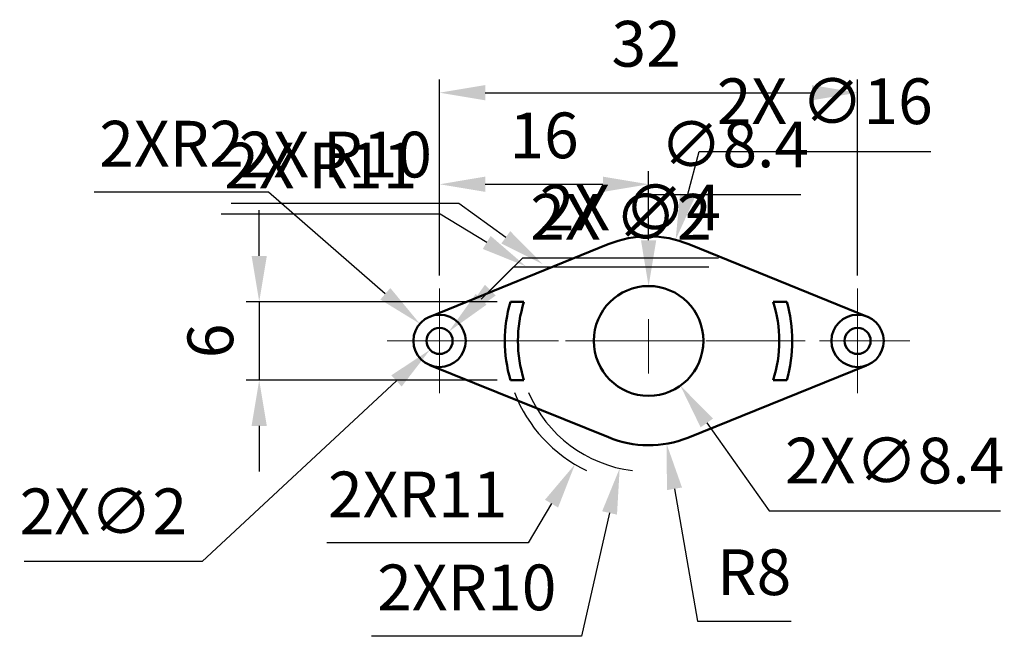
# Model space of a CAD drawing. Units: millimetres. Extents: x 788.6 to 864, y 1070.8 to 1118.
import ezdxf

# ---------------------------------------------------------------- set-up
doc = ezdxf.new("R2010")
doc.units = ezdxf.units.MM
doc.linetypes.add('CENTER', pattern=[50.8, 31.75, -6.35, 6.35, -6.35])
for name, color, linetype, lineweight in [('M-CNTR', 4, 'CENTER', 18), ('M-DIMS', 3, 'Continuous', 25), ('M-OUTL', 7, 'Continuous', 50)]:
    doc.layers.add(name, color=color, linetype=linetype, lineweight=lineweight)
doc.styles.get("Standard").update_dxf_attribs({"font": 'arial.ttf'})
doc.dimstyles.new('AM_ISO$0', dxfattribs={"dimtxt": 3.5, "dimasz": 3.5, "dimexe": 1, "dimexo": 1, "dimgap": 1.5, "dimtad": 1, "dimdsep": 46, "dimtxsty": 'Standard', "dimcen": 0, "dimclrd": 256, "dimclre": 256, "dimclrt": 2, "dimadec": 0, "dimazin": 2, "dimtp": 0.1, "dimtm": 0.1, "dimtfac": 0.71, "dimtdec": 3, "dimtmove": 0, "dimatfit": 3, "dimfxl": 1, "dimlwd": -1, "dimlwe": -1, "dimarcsym": 1})
doc.dimstyles.new('AM_ISO$3', dxfattribs={"dimtxt": 3.5, "dimasz": 3.5, "dimexe": 1, "dimexo": 1, "dimgap": 1.5, "dimtad": 1, "dimtoh": 1, "dimdsep": 46, "dimtxsty": 'Standard', "dimcen": 0, "dimclrd": 256, "dimclre": 256, "dimclrt": 2, "dimadec": 0, "dimazin": 2, "dimtp": 0.1, "dimtm": 0.1, "dimtfac": 0.71, "dimtdec": 3, "dimtofl": 0, "dimtmove": 0, "dimatfit": 0, "dimfxl": 1, "dimlwd": -1, "dimlwe": -1, "dimarcsym": 1})
doc.dimstyles.new('AM_ISO$4', dxfattribs={"dimtxt": 3.5, "dimasz": 3.5, "dimexe": 1, "dimexo": 1, "dimgap": 1.5, "dimtad": 1, "dimtoh": 1, "dimdsep": 46, "dimtxsty": 'Standard', "dimcen": 0, "dimclrd": 256, "dimclre": 256, "dimclrt": 2, "dimadec": 0, "dimazin": 2, "dimtp": 0.1, "dimtm": 0.1, "dimtfac": 0.71, "dimtdec": 3, "dimtofl": 0, "dimtmove": 0, "dimatfit": 0, "dimfxl": 1, "dimlwd": -1, "dimlwe": -1, "dimarcsym": 1})

# ---------------------------------------------------------------- blocks, each defined once
blk = doc.blocks.new('*D3')
at = {"layer": 'Defpoints', "color": 0, "transparency": 16777216}
for p in [(852.737, 1112.418), (820.737, 1097.425), (852.737, 1097.425)]:
    blk.add_point(p, dxfattribs=at)
at = {"layer": 'M-DIMS', "color": 0, "linetype": 'ByBlock', "transparency": 16777216}
for p, q in [((820.737, 1098.425), (820.737, 1113.418)), ((852.737, 1098.425), (852.737, 1113.418)), ((824.237, 1112.418), (849.237, 1112.418))]:
    blk.add_line(p, q, dxfattribs=at)
at = {"layer": 'M-DIMS', "color": 0, "transparency": 16777216}
for points in [[(824.237, 1113.002), (824.237, 1111.835), (820.737, 1112.418)], [(849.237, 1113.002), (849.237, 1111.835), (852.737, 1112.418)]]:
    blk.add_solid(points, dxfattribs=at)
at = {"layer": 'M-DIMS', "color": 0, "transparency": 16777216, "insert": (836.548, 1115.707), "char_height": 3.5, "attachment_point": 5}
blk.add_mtext('32', dxfattribs=at)
blk = doc.blocks.new('*D4')
at = {"layer": 'Defpoints', "color": 0, "transparency": 16777216}
for p in [(826.154, 1096.425), (806.929, 1090.425), (826.154, 1090.425)]:
    blk.add_point(p, dxfattribs=at)
at = {"layer": 'M-DIMS', "color": 0, "linetype": 'ByBlock', "transparency": 16777216}
for p, q in [((806.929, 1099.925), (806.929, 1103.425)), ((825.154, 1096.425), (805.929, 1096.425)), ((806.929, 1096.425), (806.929, 1090.425)), ((825.154, 1090.425), (805.929, 1090.425)), ((806.929, 1086.925), (806.929, 1083.425))]:
    blk.add_line(p, q, dxfattribs=at)
at = {"layer": 'M-DIMS', "color": 0, "transparency": 16777216}
for points in [[(806.346, 1099.925), (807.513, 1099.925), (806.929, 1096.425)], [(806.346, 1086.925), (807.513, 1086.925), (806.929, 1090.425)]]:
    blk.add_solid(points, dxfattribs=at)
at = {"layer": 'M-DIMS', "color": 0, "transparency": 16777216, "insert": (803.642, 1093.425), "char_height": 3.5, "attachment_point": 5, "rotation": 90}
blk.add_mtext('6', dxfattribs=at)
blk = doc.blocks.new('*D5')
at = {"layer": 'Defpoints', "color": 0, "transparency": 16777216}
for p in [(819.227, 1094.737), (820.737, 1093.425)]:
    blk.add_point(p, dxfattribs=at)
at = {"layer": 'M-DIMS', "color": 0, "linetype": 'ByBlock', "transparency": 16777216}
for p, q in [((807.633, 1104.805), (794.303, 1104.805)), ((816.584, 1097.032), (807.633, 1104.805))]:
    blk.add_line(p, q, dxfattribs=at)
at = {"layer": 'M-DIMS', "color": 0, "transparency": 16777216}
blk.add_solid([(816.967, 1097.472), (816.202, 1096.591), (819.227, 1094.737)], dxfattribs=at)
at = {"layer": 'M-DIMS', "color": 0, "transparency": 16777216, "insert": (800.218, 1108.062), "char_height": 3.5, "attachment_point": 5}
blk.add_mtext('2XR2', dxfattribs=at)
blk = doc.blocks.new('*D6')
at = {"layer": 'Defpoints', "color": 0, "transparency": 16777216}
for p in [(836.737, 1093.425), (831.101, 1083.979)]:
    blk.add_point(p, dxfattribs=at)
at = {"layer": 'M-DIMS', "color": 0, "linetype": 'ByBlock', "transparency": 16777216}
for p, q in [((829.308, 1080.973), (827.515, 1077.967)), ((827.515, 1077.967), (812.106, 1077.967))]:
    blk.add_line(p, q, dxfattribs=at)
blk.add_arc((836.737, 1093.425), 11, 201.03533, 244.39114, dxfattribs=at)
at = {"layer": 'M-DIMS', "color": 0, "transparency": 16777216}
blk.add_solid([(828.807, 1081.272), (829.809, 1080.674), (831.101, 1083.979)], dxfattribs=at)
at = {"layer": 'M-DIMS', "color": 0, "transparency": 16777216, "insert": (819.061, 1081.224), "char_height": 3.5, "attachment_point": 5}
blk.add_mtext('2XR11', dxfattribs=at)
blk = doc.blocks.new('*D7')
at = {"layer": 'Defpoints', "color": 0, "transparency": 16777216}
for p in [(836.737, 1093.425), (834.524, 1083.673)]:
    blk.add_point(p, dxfattribs=at)
at = {"layer": 'M-DIMS', "color": 0, "linetype": 'ByBlock', "transparency": 16777216}
for p, q in [((833.75, 1080.26), (831.608, 1070.823)), ((831.608, 1070.823), (815.535, 1070.823))]:
    blk.add_line(p, q, dxfattribs=at)
blk.add_arc((836.737, 1093.425), 10, 203.18718, 262.9463, dxfattribs=at)
at = {"layer": 'M-DIMS', "color": 0, "transparency": 16777216}
blk.add_solid([(833.181, 1080.389), (834.319, 1080.131), (834.524, 1083.673)], dxfattribs=at)
at = {"layer": 'M-DIMS', "color": 0, "transparency": 16777216, "insert": (822.822, 1074.11), "char_height": 3.5, "attachment_point": 5}
blk.add_mtext('2XR10', dxfattribs=at)
blk = doc.blocks.new('*D8')
at = {"layer": 'Defpoints', "color": 0, "transparency": 16777216}
for p in [(836.737, 1093.436), (838.116, 1085.556)]:
    blk.add_point(p, dxfattribs=at)
at = {"layer": 'M-DIMS', "color": 0, "linetype": 'ByBlock', "transparency": 16777216}
for p, q in [((838.719, 1082.109), (840.49, 1071.986)), ((840.49, 1071.986), (847.641, 1071.986))]:
    blk.add_line(p, q, dxfattribs=at)
at = {"layer": 'M-DIMS', "color": 0, "transparency": 16777216}
blk.add_solid([(839.294, 1082.209), (838.144, 1082.008), (838.116, 1085.556)], dxfattribs=at)
at = {"layer": 'M-DIMS', "color": 0, "transparency": 16777216, "insert": (844.816, 1075.273), "char_height": 3.5, "attachment_point": 5}
blk.add_mtext('R8', dxfattribs=at)
blk = doc.blocks.new('*D9')
at = {"layer": 'Defpoints', "color": 0, "transparency": 16777216}
for p in [(821.47, 1094.106), (820.004, 1092.745)]:
    blk.add_point(p, dxfattribs=at)
at = {"layer": 'M-DIMS', "color": 0, "linetype": 'ByBlock', "transparency": 16777216}
for p, q in [((817.438, 1090.364), (802.55, 1076.546)), ((802.55, 1076.546), (788.948, 1076.546))]:
    blk.add_line(p, q, dxfattribs=at)
at = {"layer": 'M-DIMS', "color": 0, "transparency": 16777216}
blk.add_solid([(817.042, 1090.792), (817.835, 1089.937), (820.004, 1092.745)], dxfattribs=at)
at = {"layer": 'M-DIMS', "color": 0, "transparency": 16777216, "insert": (794.999, 1079.931), "char_height": 3.5, "attachment_point": 5}
blk.add_mtext('2X∅2', dxfattribs=at)
blk = doc.blocks.new('*D10')
at = {"layer": 'Defpoints', "color": 0, "transparency": 16777216}
for p in [(834.303, 1096.849), (839.17, 1090.002)]:
    blk.add_point(p, dxfattribs=at)
at = {"layer": 'M-DIMS', "color": 0, "linetype": 'ByBlock', "transparency": 16777216}
for p, q in [((841.198, 1087.149), (845.974, 1080.429)), ((845.974, 1080.429), (863.676, 1080.429))]:
    blk.add_line(p, q, dxfattribs=at)
at = {"layer": 'M-DIMS', "color": 0, "transparency": 16777216}
blk.add_solid([(841.673, 1087.487), (840.722, 1086.811), (839.17, 1090.002)], dxfattribs=at)
at = {"layer": 'M-DIMS', "color": 0, "transparency": 16777216, "insert": (855.575, 1083.814), "char_height": 3.5, "attachment_point": 5}
blk.add_mtext('2X∅8.4', dxfattribs=at)
blk = doc.blocks.new('PLATE-END-EYE')
for radius in [2, 1]:
    blk.add_circle((0, 0), radius)
blk = doc.blocks.new('PLATE-ARC-SLOT')
for p, q in [((-0.083, 3), (0.961, 3)), ((-0.083, -3), (0.961, -3))]:
    blk.add_line(p, q)
for radius, start, end in [(11, 164.17338, 195.82662), (10, 162.5424, 197.4576)]:
    blk.add_arc((10.5, 0), radius, start, end)
blk = doc.blocks.new('*D13')
at = {"layer": 'Defpoints', "color": 0, "transparency": 16777216}
for p in [(836.737, 1105.411), (836.737, 1101.436), (820.737, 1097.425)]:
    blk.add_point(p, dxfattribs=at)
at = {"layer": 'M-DIMS', "linetype": 'ByBlock', "transparency": 16777216}
for p, q in [((820.737, 1098.425), (820.737, 1106.411)), ((836.737, 1102.436), (836.737, 1106.411)), ((824.237, 1105.411), (833.237, 1105.411))]:
    blk.add_line(p, q, dxfattribs=at)
at = {"layer": 'M-DIMS', "transparency": 16777216}
for points in [[(824.237, 1105.995), (824.237, 1104.828), (820.737, 1105.411)], [(833.237, 1105.995), (833.237, 1104.828), (836.737, 1105.411)]]:
    blk.add_solid(points, dxfattribs=at)
at = {"layer": 'M-DIMS', "color": 2, "transparency": 16777216, "insert": (828.737, 1108.698), "char_height": 3.5, "attachment_point": 5}
blk.add_mtext('16', dxfattribs=at)
blk = doc.blocks.new('*D14')
at = {"layer": 'Defpoints', "color": 0, "transparency": 16777216}
for p in [(822.151, 1094.839), (819.322, 1092.012)]:
    blk.add_point(p, dxfattribs=at)
at = {"layer": 'M-DIMS', "linetype": 'ByBlock', "transparency": 16777216}
for p, q in [((824.627, 1097.314), (827.102, 1099.788)), ((827.102, 1099.788), (842.084, 1099.788))]:
    blk.add_line(p, q, dxfattribs=at)
at = {"layer": 'M-DIMS', "transparency": 16777216}
blk.add_solid([(824.214, 1097.726), (825.039, 1096.901), (822.151, 1094.839)], dxfattribs=at)
at = {"layer": 'M-DIMS', "color": 2, "transparency": 16777216, "insert": (835.343, 1103.173), "char_height": 3.5, "attachment_point": 5}
blk.add_mtext('2X ∅4', dxfattribs=at)
blk = doc.blocks.new('*D15')
at = {"layer": 'Defpoints', "color": 0, "transparency": 16777216}
for p in [(821.444, 1094.133), (820.03, 1092.718)]:
    blk.add_point(p, dxfattribs=at)
at = {"layer": 'M-DIMS', "linetype": 'ByBlock', "transparency": 16777216}
for p, q in [((823.918, 1096.608), (826.392, 1099.083)), ((826.392, 1099.083), (841.353, 1099.083))]:
    blk.add_line(p, q, dxfattribs=at)
at = {"layer": 'M-DIMS', "transparency": 16777216}
blk.add_solid([(823.506, 1097.02), (824.331, 1096.196), (821.444, 1094.133)], dxfattribs=at)
at = {"layer": 'M-DIMS', "color": 2, "transparency": 16777216, "insert": (834.623, 1102.468), "char_height": 3.5, "attachment_point": 5}
blk.add_mtext('2X ∅2', dxfattribs=at)
blk = doc.blocks.new('*D16')
at = {"layer": 'Defpoints', "color": 0, "transparency": 16777216}
for p in [(836.737, 1097.625), (836.736, 1089.225)]:
    blk.add_point(p, dxfattribs=at)
at = {"layer": 'M-DIMS', "linetype": 'ByBlock', "transparency": 16777216}
for p, q in [((836.737, 1101.125), (836.737, 1104.625)), ((836.737, 1104.625), (848.403, 1104.625))]:
    blk.add_line(p, q, dxfattribs=at)
at = {"layer": 'M-DIMS', "transparency": 16777216}
blk.add_solid([(836.154, 1101.125), (837.321, 1101.125), (836.737, 1097.625)], dxfattribs=at)
at = {"layer": 'M-DIMS', "color": 2, "transparency": 16777216, "insert": (843.32, 1108.01), "char_height": 3.5, "attachment_point": 5}
blk.add_mtext('∅8.4', dxfattribs=at)
blk = doc.blocks.new('*D17')
at = {"layer": 'Defpoints', "color": 0, "transparency": 16777216}
for p in [(838.807, 1101.164), (834.667, 1085.709)]:
    blk.add_point(p, dxfattribs=at)
at = {"layer": 'M-DIMS', "linetype": 'ByBlock', "transparency": 16777216}
for p, q in [((839.713, 1104.545), (840.618, 1107.925)), ((840.618, 1107.925), (858.332, 1107.925))]:
    blk.add_line(p, q, dxfattribs=at)
at = {"layer": 'M-DIMS', "transparency": 16777216}
blk.add_solid([(839.149, 1104.696), (840.276, 1104.394), (838.807, 1101.164)], dxfattribs=at)
at = {"layer": 'M-DIMS', "color": 2, "transparency": 16777216, "insert": (850.225, 1111.31), "char_height": 3.5, "attachment_point": 5}
blk.add_mtext('2X ∅16', dxfattribs=at)
blk = doc.blocks.new('*D18')
at = {"layer": 'Defpoints', "color": 0, "transparency": 16777216}
for p in [(827.337, 1099.139), (836.737, 1093.425)]:
    blk.add_point(p, dxfattribs=at)
at = {"layer": 'M-DIMS', "linetype": 'ByBlock', "transparency": 16777216}
for p, q in [((820.777, 1103.127), (804.01, 1103.127)), ((824.346, 1100.957), (820.777, 1103.127))]:
    blk.add_line(p, q, dxfattribs=at)
at = {"layer": 'M-DIMS', "transparency": 16777216}
blk.add_solid([(824.649, 1101.456), (824.043, 1100.459), (827.337, 1099.139)], dxfattribs=at)
at = {"layer": 'M-DIMS', "color": 2, "transparency": 16777216, "insert": (811.643, 1106.385), "char_height": 3.5, "attachment_point": 5}
blk.add_mtext('2X R11', dxfattribs=at)
blk = doc.blocks.new('*D19')
at = {"layer": 'Defpoints', "color": 0, "transparency": 16777216}
for p in [(828.639, 1099.293), (836.737, 1093.425)]:
    blk.add_point(p, dxfattribs=at)
at = {"layer": 'M-DIMS', "linetype": 'ByBlock', "transparency": 16777216}
for p, q in [((822.223, 1103.942), (804.791, 1103.942)), ((825.805, 1101.346), (822.223, 1103.942))]:
    blk.add_line(p, q, dxfattribs=at)
at = {"layer": 'M-DIMS', "transparency": 16777216}
blk.add_solid([(826.147, 1101.819), (825.462, 1100.874), (828.639, 1099.293)], dxfattribs=at)
at = {"layer": 'M-DIMS', "color": 2, "transparency": 16777216, "insert": (812.757, 1107.229), "char_height": 3.5, "attachment_point": 5}
blk.add_mtext('2X R10', dxfattribs=at)

msp = doc.modelspace()

# ---------------------------------------------------------------- linework, layer by layer
at = {"layer": 'M-CNTR'}
for p, q in [((820.737, 1089.425), (820.737, 1097.425)), ((852.737, 1089.425), (852.737, 1097.425)), ((836.737, 1090.924), (836.737, 1095.077)), ((816.737, 1093.425), (829.85, 1093.425)), ((830.369, 1093.425), (840.937, 1093.425)), ((841.11, 1093.425), (848.737, 1093.425)), ((849.812, 1093.425), (856.737, 1093.425))]:
    msp.add_line(p, q, dxfattribs=at)
at = {"layer": 'M-OUTL'}
for p, q in [((833.654, 1100.819), (819.986, 1095.279)), ((839.819, 1100.819), (853.488, 1095.279)), ((833.665, 1086.05), (819.988, 1091.571)), ((853.424, 1091.547), (839.732, 1086.018))]:
    msp.add_line(p, q, dxfattribs=at)
msp.add_circle((836.737, 1093.425), 4.2, dxfattribs=at)
for start, end in [(67.33881, 112.66119), (247.42147, 291.98928)]:
    msp.add_arc((836.737, 1093.436), 8, start, end, dxfattribs=at)

# ---------------------------------------------------------------- block references
for name, p in [('PLATE-ARC-SLOT', (826.237, 1093.425)), ('PLATE-END-EYE', (820.737, 1093.425)), ('PLATE-END-EYE', (852.737, 1093.425))]:
    msp.add_blockref(name, p, dxfattribs=at)
at = {"layer": 'M-OUTL', "rotation": 180}
msp.add_blockref('PLATE-ARC-SLOT', (847.237, 1093.425), dxfattribs=at)

# ---------------------------------------------------------------- dimensions: what is measured, and where the dimension line sits
at = {"layer": 'M-DIMS'}
dim = msp.add_linear_dim(base=(852.737, 1112.418), p1=(820.737, 1097.425), p2=(852.737, 1097.425), dimstyle='AM_ISO$0', override={"dimclrd": 0, "dimclre": 0, "dimclrt": 0}, dxfattribs=at)
dim.commit()
dim.dimension.update_dxf_attribs({"geometry": '*D3', "text_midpoint": (836.548, 1112.418), "dimtype": 160})
for p1, p2, text, dimstyle, override, picture, middle in [((834.667, 1085.709), (838.807, 1101.164), '2X <>', 'AM_ISO$4', {"dimdec": 0, "dimlfac": 1, "dimrnd": 0, "dimzin": 0, "dimdsep": 46, "dimlunit": 2}, '*D17', (850.225, 1107.925)), ((819.322, 1092.012), (822.151, 1094.839), '2X <>', 'AM_ISO$4', {"dimdec": 0, "dimlfac": 1, "dimrnd": 0, "dimzin": 0, "dimdsep": 46, "dimlunit": 2}, '*D14', (835.343, 1099.788)), ((820.03, 1092.718), (821.444, 1094.133), '2X <>', 'AM_ISO$4', {"dimdec": 0, "dimlfac": 1, "dimrnd": 0, "dimzin": 0, "dimdsep": 46, "dimlunit": 2}, '*D15', (834.623, 1099.083)), ((834.303, 1096.849), (839.17, 1090.002), '2X<>', 'AM_ISO$3', {"dimpost": '', "dimclrd": 0, "dimclre": 0, "dimclrt": 0}, '*D10', (855.575, 1080.429)), ((821.47, 1094.106), (820.004, 1092.745), '2X<>', 'AM_ISO$3', {"dimclrd": 0, "dimclre": 0, "dimclrt": 0}, '*D9', (794.999, 1076.546))]:
    dim = msp.add_diameter_dim_2p(p1=p1, p2=p2, text=text, dimstyle=dimstyle, override=override, dxfattribs=at)
    dim.commit()
    dim.dimension.update_dxf_attribs({"geometry": picture, "text_midpoint": middle, "dimtype": 163})
for center, mpoint, text, override, picture, middle in [((836.737, 1093.425), (828.639, 1099.293), '2X <>', {"dimdec": 0, "dimlfac": 1, "dimrnd": 0, "dimzin": 0, "dimdsep": 46, "dimlunit": 2}, '*D19', (812.757, 1103.942)), ((836.737, 1093.425), (827.337, 1099.139), '2X <>', {"dimdec": 0, "dimlfac": 1, "dimrnd": 0, "dimzin": 0, "dimdsep": 46, "dimlunit": 2}, '*D18', (811.643, 1103.127)), ((820.737, 1093.425), (819.227, 1094.737), '2X<>', {"dimclrd": 0, "dimclre": 0, "dimclrt": 0}, '*D5', (800.218, 1104.805)), ((836.737, 1093.425), (831.101, 1083.979), '2X<>', {"dimpost": '', "dimclrd": 0, "dimclre": 0, "dimclrt": 0}, '*D6', (819.061, 1077.967)), ((836.737, 1093.425), (834.524, 1083.673), '2X<>', {"dimpost": '', "dimclrd": 0, "dimclre": 0, "dimclrt": 0}, '*D7', (822.822, 1070.823))]:
    dim = msp.add_radius_dim(center=center, mpoint=mpoint, text=text, dimstyle='AM_ISO$4', override=override, dxfattribs=at)
    dim.commit()
    dim.dimension.update_dxf_attribs({"geometry": picture, "text_midpoint": middle, "dimtype": 164})
dim = msp.add_linear_dim(base=(836.737, 1105.411), p1=(820.737, 1097.425), p2=(836.737, 1101.436), dimstyle='AM_ISO$4', override={"dimdec": 0, "dimlfac": 1, "dimrnd": 0, "dimzin": 0, "dimdsep": 46, "dimlunit": 2}, dxfattribs=at)
dim.commit()
dim.dimension.update_dxf_attribs({"geometry": '*D13', "text_midpoint": (828.737, 1108.698)})
dim = msp.add_diameter_dim_2p(p1=(836.736, 1089.225), p2=(836.737, 1097.625), dimstyle='AM_ISO$4', override={"dimdec": 1, "dimlfac": 1, "dimrnd": 0, "dimzin": 0, "dimdsep": 46, "dimlunit": 2}, dxfattribs=at)
dim.commit()
dim.dimension.update_dxf_attribs({"geometry": '*D16', "text_midpoint": (843.32, 1104.625), "dimtype": 163})
dim = msp.add_linear_dim(base=(806.929, 1090.425), p1=(826.154, 1096.425), p2=(826.154, 1090.425), angle=90, dimstyle='AM_ISO$0', override={"dimclrd": 0, "dimclre": 0, "dimclrt": 0}, dxfattribs=at)
dim.commit()
dim.dimension.update_dxf_attribs({"geometry": '*D4', "text_midpoint": (806.929, 1093.425), "dimtype": 160})
dim = msp.add_radius_dim(center=(836.737, 1093.436), mpoint=(838.116, 1085.556), dimstyle='AM_ISO$4', override={"dimclrd": 0, "dimclre": 0, "dimclrt": 0}, dxfattribs=at)
dim.commit()
dim.dimension.update_dxf_attribs({"geometry": '*D8', "text_midpoint": (844.816, 1071.986), "dimtype": 164})

doc.saveas('drawing.dxf')
